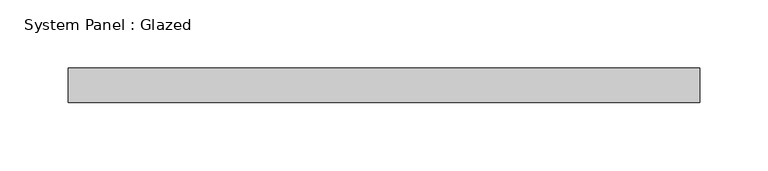
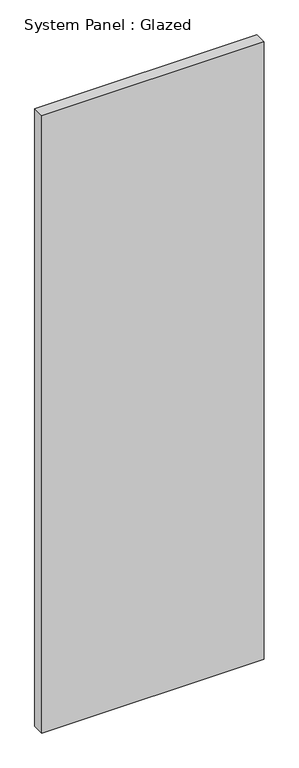
"""IFC4 building model written with IfcOpenShell, lengths in millimetres: plate geometry, System Panel : Glazed."""

from ifc_helpers import new_model, si_unit, origin, origin_with_axes, place, context, project, spatial, polyline, outline, extrude, source, transform, mapped, element, save


def system_panel_glazed_5b9b0e9e(model_context):
    return source(origin(), model_context, "Body", "SweptSolid", [
        extrude(outline(polyline([(231.775, 19.05), (-231.775, 19.05), (-231.775, 44.45), (231.775, 44.45), (231.775, 19.05)])), origin_with_axes(), (0.0, 0.0, 1.0), 1359.8504732),
    ])


if __name__ == "__main__":
    model = new_model("IFC4")
    model_context = context("Model", 3, world=origin())
    ifc_project = project(units=[si_unit("LENGTHUNIT", "METRE", prefix="MILLI")], contexts=[model_context])
    site = spatial("IfcSite", under=ifc_project)
    building = spatial("IfcBuilding", under=site)
    placement = place(None, origin())
    system_panel_glazed_shape = system_panel_glazed_5b9b0e9e(model_context)
    element("IfcPlate", 1, ObjectType="System Panel : Glazed", at=placement, inside=building, context=model_context, shape_type="MappedRepresentation", body=[
        mapped(system_panel_glazed_shape, transform((0.0, 0.0, 0.0), x_axis=(1.0, 0.0, 0.0), y_axis=(0.0, 1.0, 0.0), z_axis=(0.0, 0.0, 1.0))),
    ])
    save(model, "model.ifc")

# Revit data of these elements
# Type "System Panel : Glazed"
#   Construction Type Id = "GSP4R"
#   Analytic Construction = "1/8 in Pilkington single glazing"
#   Visual Light Transmittance = 0.9
#   Solar Heat Gain Coefficient = 0.86
#   Heat Transfer Coefficient (U) = 1.18115 BTU/(h·ft²·°F)
#   Define Thermal Properties by = 1
# Element 1 (IfcPlate, "System Panel : Glazed")
#   Materials on its faces: "Glass"
# Materials
#   "Glass": class "Glass", colour RGB 0 128 192, transparency 0.75, Description = "Soda Lime Glass", Cost = 0
